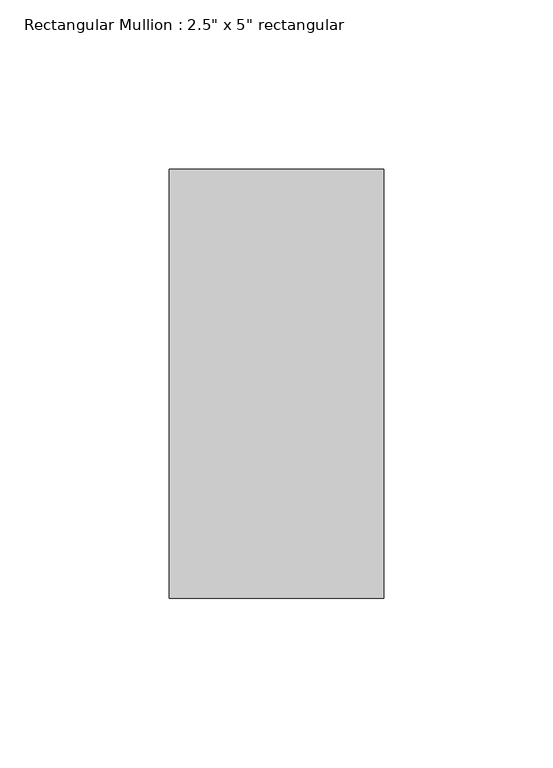
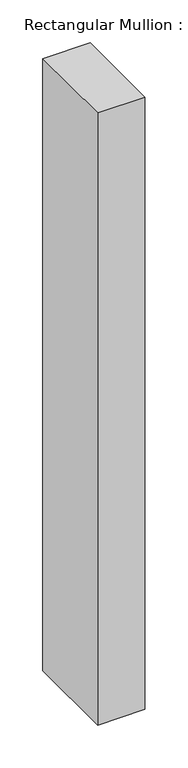
"""IFC4 building model written with IfcOpenShell, lengths in millimetres: member geometry."""

from ifc_helpers import new_model, si_unit, frame, origin, place, context, project, spatial, polyline, outline, extrude, source, transform, mapped, element, save


def member_024c663a(model_context):
    return source(origin(), model_context, "Body", "SweptSolid", [
        extrude(outline(polyline([(0.0, 63.5), (0.0, -63.5), (-63.5, -63.5), (-63.5, 63.5), (0.0, 63.5)])), frame((0.0, 0.0, -869.95), z_axis=(0.0, 0.0, 1.0), x_axis=(1.0, 0.0, 0.0)), (0.0, 0.0, 1.0), 869.95),
    ])


if __name__ == "__main__":
    model = new_model("IFC4")
    model_context = context("Model", 3, world=origin())
    ifc_project = project(units=[si_unit("LENGTHUNIT", "METRE", prefix="MILLI")], contexts=[model_context])
    site = spatial("IfcSite", under=ifc_project)
    building = spatial("IfcBuilding", under=site)
    placement = place(None, origin())
    member_shape = member_024c663a(model_context)
    element("IfcMember", 1, ObjectType="Rectangular Mullion : 2.5\" x 5\" rectangular", at=placement, inside=building, context=model_context, shape_type="MappedRepresentation", body=[
        mapped(member_shape, transform((0.0, 0.0, 0.0), x_axis=(1.0, 0.0, 0.0), y_axis=(0.0, 1.0, 0.0), z_axis=(0.0, 0.0, 1.0))),
    ])
    save(model, "model.ifc")

# Revit data of these elements
# Type "Rectangular Mullion : 2.5\" x 5\" rectangular"
#   built-in parameter 1007304 = 0.416667 (stored number, unit not read)
#   built-in parameter 1007301 = 0.104167 (stored number, unit not read)
#   built-in parameter 1007300 = 0.104167 (stored number, unit not read)
# Element 1 (IfcMember, "Rectangular Mullion : 2.5\" x 5\" rectangular")
#   Materials on its faces: "Aluminum"
# Materials
#   "Aluminum": class "Metal", colour RGB 247 247 247, transparency 0, Description = "Aluminum 6061", Cost = 0
